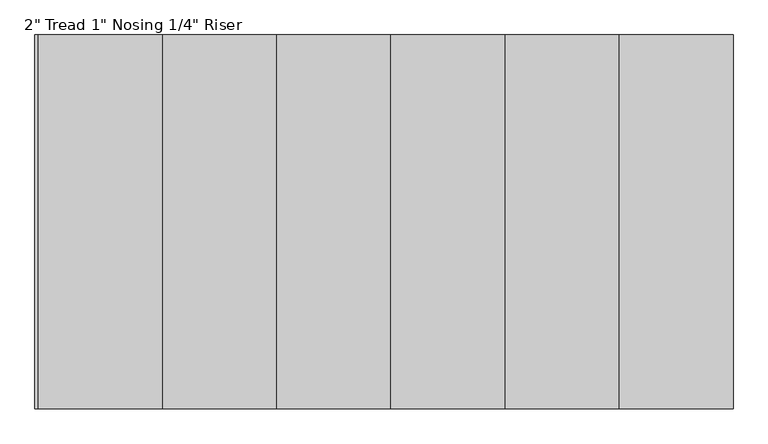
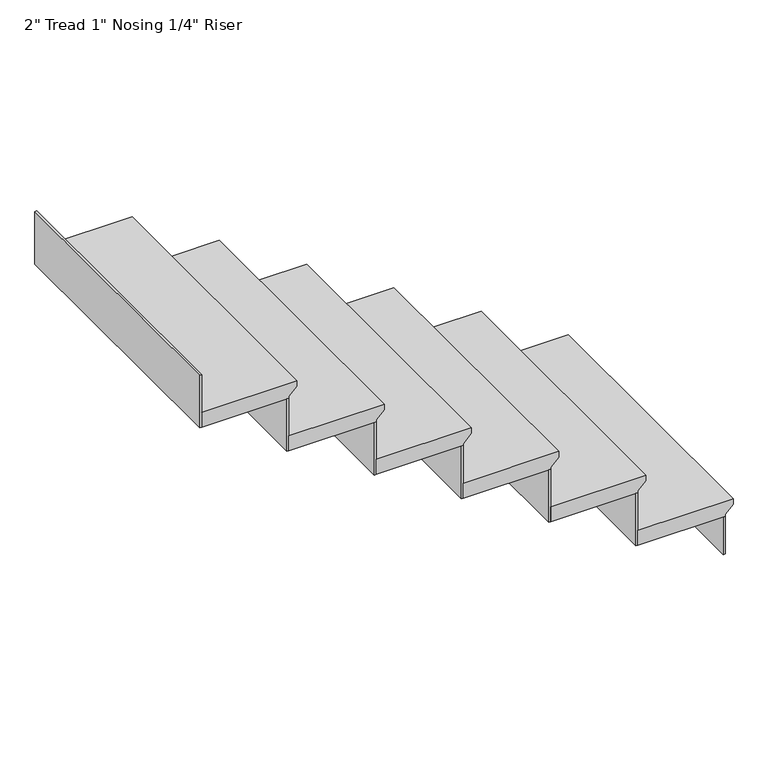
"""IFC4 building model written with IfcOpenShell, lengths in millimetres: stair flight geometry."""

from ifc_helpers import new_model, si_unit, origin, place, context, project, spatial, faceted_brep, source, transform, mapped, element, save


def stair_flight_b9929406(model_context):
    return source(origin(), model_context, "Body", "Brep", [
        faceted_brep([(-6576.0763529, -1051.6338022, 7169.15), (-6576.0763529, -1051.6338022, 7188.2), (-6576.0763529, -1966.0338022, 7188.2), (-6576.0763529, -1966.0338022, 7169.15), (-6601.4763529, -1051.6338022, 7143.75), (-6601.4763529, -1966.0338022, 7143.75), (-6880.8763529, -1051.6338022, 7188.2), (-6880.8763529, -1966.0338022, 7188.2), (-6601.4763529, -1966.0338022, 7137.4), (-6880.8763529, -1966.0338022, 7137.4), (-6880.8763529, -1051.6338022, 7137.4), (-6601.4763529, -1051.6338022, 7137.4)], [[[0, 1, 2, 3]], [[4, 0, 3, 5]], [[2, 1, 6, 7]], [[8, 9, 10, 11]], [[2, 7, 9, 8, 5, 3]], [[8, 11, 4, 5]], [[6, 1, 0, 4, 11, 10]], [[7, 6, 10, 9]]]),
        faceted_brep([(-6601.4763529, -1051.6338022, 7137.4), (-6601.4763529, -1051.6338022, 7010.4), (-6607.8263529, -1051.6338022, 7010.4), (-6607.8263529, -1051.6338022, 7137.4), (-6601.4763529, -1966.0338022, 7137.4), (-6607.8263529, -1966.0338022, 7137.4), (-6607.8263529, -1966.0338022, 7010.4), (-6601.4763529, -1966.0338022, 7010.4)], [[[0, 1, 2, 3]], [[4, 5, 6, 7]], [[1, 0, 4, 7]], [[2, 1, 7, 6]], [[3, 2, 6, 5]], [[0, 3, 5, 4]]]),
        faceted_brep([(-6880.8763529, -1051.6338022, 7315.2), (-6880.8763529, -1051.6338022, 7137.4), (-6887.2263529, -1051.6338022, 7137.4), (-6887.2263529, -1051.6338022, 7315.2), (-6880.8763529, -1966.0338022, 7315.2), (-6887.2263529, -1966.0338022, 7315.2), (-6887.2263529, -1966.0338022, 7137.4), (-6880.8763529, -1966.0338022, 7137.4)], [[[0, 1, 2, 3]], [[4, 5, 6, 7]], [[1, 0, 4, 7]], [[2, 1, 7, 6]], [[3, 2, 6, 5]], [[0, 3, 5, 4]]]),
        faceted_brep([(-6855.4763529, -1966.0338022, 7366.0), (-6855.4763529, -1051.6338022, 7366.0), (-7160.2763529, -1051.6338022, 7366.0), (-7160.2763529, -1966.0338022, 7366.0), (-6880.8763529, -1966.0338022, 7315.2), (-7160.2763529, -1966.0338022, 7315.2), (-7160.2763529, -1051.6338022, 7315.2), (-6880.8763529, -1051.6338022, 7315.2), (-6880.8763529, -1966.0338022, 7321.55), (-6855.4763529, -1966.0338022, 7346.95), (-6880.8763529, -1051.6338022, 7321.55), (-6855.4763529, -1051.6338022, 7346.95)], [[[0, 1, 2, 3]], [[4, 5, 6, 7]], [[0, 3, 5, 4, 8, 9]], [[4, 7, 10, 8]], [[2, 1, 11, 10, 7, 6]], [[3, 2, 6, 5]], [[11, 1, 0, 9]], [[10, 11, 9, 8]]]),
        faceted_brep([(-7160.2763529, -1051.6338022, 7493.0), (-7160.2763529, -1051.6338022, 7315.2), (-7166.6263529, -1051.6338022, 7315.2), (-7166.6263529, -1051.6338022, 7493.0), (-7160.2763529, -1966.0338022, 7493.0), (-7166.6263529, -1966.0338022, 7493.0), (-7166.6263529, -1966.0338022, 7315.2), (-7160.2763529, -1966.0338022, 7315.2)], [[[0, 1, 2, 3]], [[4, 5, 6, 7]], [[1, 0, 4, 7]], [[2, 1, 7, 6]], [[3, 2, 6, 5]], [[0, 3, 5, 4]]]),
        faceted_brep([(-7134.8763529, -1966.0338022, 7543.8), (-7134.8763529, -1051.6338022, 7543.8), (-7439.6763529, -1051.6338022, 7543.8), (-7439.6763529, -1966.0338022, 7543.8), (-7160.2763529, -1966.0338022, 7493.0), (-7439.6763529, -1966.0338022, 7493.0), (-7439.6763529, -1051.6338022, 7493.0), (-7160.2763529, -1051.6338022, 7493.0), (-7160.2763529, -1966.0338022, 7499.35), (-7134.8763529, -1966.0338022, 7524.75), (-7160.2763529, -1051.6338022, 7499.35), (-7134.8763529, -1051.6338022, 7524.75)], [[[0, 1, 2, 3]], [[4, 5, 6, 7]], [[0, 3, 5, 4, 8, 9]], [[4, 7, 10, 8]], [[2, 1, 11, 10, 7, 6]], [[3, 2, 6, 5]], [[11, 1, 0, 9]], [[10, 11, 9, 8]]]),
        faceted_brep([(-7439.6763529, -1051.6338022, 7670.8), (-7439.6763529, -1051.6338022, 7493.0), (-7446.0263529, -1051.6338022, 7493.0), (-7446.0263529, -1051.6338022, 7670.8), (-7439.6763529, -1966.0338022, 7670.8), (-7446.0263529, -1966.0338022, 7670.8), (-7446.0263529, -1966.0338022, 7493.0), (-7439.6763529, -1966.0338022, 7493.0)], [[[0, 1, 2, 3]], [[4, 5, 6, 7]], [[1, 0, 4, 7]], [[2, 1, 7, 6]], [[3, 2, 6, 5]], [[0, 3, 5, 4]]]),
        faceted_brep([(-7414.2763529, -1966.0338022, 7721.6), (-7414.2763529, -1051.6338022, 7721.6), (-7719.0763529, -1051.6338022, 7721.6), (-7719.0763529, -1966.0338022, 7721.6), (-7439.6763529, -1966.0338022, 7670.8), (-7719.0763529, -1966.0338022, 7670.8), (-7719.0763529, -1051.6338022, 7670.8), (-7439.6763529, -1051.6338022, 7670.8), (-7439.6763529, -1966.0338022, 7677.15), (-7414.2763529, -1966.0338022, 7702.55), (-7439.6763529, -1051.6338022, 7677.15), (-7414.2763529, -1051.6338022, 7702.55)], [[[0, 1, 2, 3]], [[4, 5, 6, 7]], [[0, 3, 5, 4, 8, 9]], [[4, 7, 10, 8]], [[2, 1, 11, 10, 7, 6]], [[3, 2, 6, 5]], [[11, 1, 0, 9]], [[10, 11, 9, 8]]]),
        faceted_brep([(-7719.0763529, -1051.6338022, 7848.6), (-7719.0763529, -1051.6338022, 7670.8), (-7725.4263529, -1051.6338022, 7670.8), (-7725.4263529, -1051.6338022, 7848.6), (-7719.0763529, -1966.0338022, 7848.6), (-7725.4263529, -1966.0338022, 7848.6), (-7725.4263529, -1966.0338022, 7670.8), (-7719.0763529, -1966.0338022, 7670.8)], [[[0, 1, 2, 3]], [[4, 5, 6, 7]], [[1, 0, 4, 7]], [[2, 1, 7, 6]], [[3, 2, 6, 5]], [[0, 3, 5, 4]]]),
        faceted_brep([(-7693.6763529, -1966.0338022, 7899.4), (-7693.6763529, -1051.6338022, 7899.4), (-7998.4763529, -1051.6338022, 7899.4), (-7998.4763529, -1966.0338022, 7899.4), (-7719.0763529, -1966.0338022, 7848.6), (-7998.4763529, -1966.0338022, 7848.6), (-7998.4763529, -1051.6338022, 7848.6), (-7719.0763529, -1051.6338022, 7848.6), (-7719.0763529, -1966.0338022, 7854.95), (-7693.6763529, -1966.0338022, 7880.35), (-7719.0763529, -1051.6338022, 7854.95), (-7693.6763529, -1051.6338022, 7880.35)], [[[0, 1, 2, 3]], [[4, 5, 6, 7]], [[0, 3, 5, 4, 8, 9]], [[4, 7, 10, 8]], [[2, 1, 11, 10, 7, 6]], [[3, 2, 6, 5]], [[11, 1, 0, 9]], [[10, 11, 9, 8]]]),
        faceted_brep([(-8277.8763529, -1051.6338022, 8204.2), (-8277.8763529, -1051.6338022, 8026.4), (-8284.2263529, -1051.6338022, 8026.4), (-8284.2263529, -1051.6338022, 8204.2), (-8277.8763529, -1966.0338022, 8204.2), (-8284.2263529, -1966.0338022, 8204.2), (-8284.2263529, -1966.0338022, 8026.4), (-8277.8763529, -1966.0338022, 8026.4)], [[[0, 1, 2, 3]], [[4, 5, 6, 7]], [[1, 0, 4, 7]], [[2, 1, 7, 6]], [[3, 2, 6, 5]], [[0, 3, 5, 4]]]),
        faceted_brep([(-7998.4763529, -1051.6338022, 8026.4), (-7998.4763529, -1051.6338022, 7848.6), (-8004.8263529, -1051.6338022, 7848.6), (-8004.8263529, -1051.6338022, 8026.4), (-7998.4763529, -1966.0338022, 8026.4), (-8004.8263529, -1966.0338022, 8026.4), (-8004.8263529, -1966.0338022, 7848.6), (-7998.4763529, -1966.0338022, 7848.6)], [[[0, 1, 2, 3]], [[4, 5, 6, 7]], [[1, 0, 4, 7]], [[2, 1, 7, 6]], [[3, 2, 6, 5]], [[0, 3, 5, 4]]]),
        faceted_brep([(-7973.0763529, -1966.0338022, 8077.2), (-7973.0763529, -1051.6338022, 8077.2), (-8252.4763529, -1051.6338022, 8077.2), (-8277.8763529, -1051.6338022, 8077.2), (-8277.8763529, -1966.0338022, 8077.2), (-7998.4763529, -1966.0338022, 8026.4), (-8277.8763529, -1966.0338022, 8026.4), (-8277.8763529, -1051.6338022, 8026.4), (-8252.4763529, -1051.6338022, 8026.4), (-7998.4763529, -1051.6338022, 8026.4), (-7998.4763529, -1966.0338022, 8032.75), (-7973.0763529, -1966.0338022, 8058.15), (-7998.4763529, -1051.6338022, 8032.75), (-7973.0763529, -1051.6338022, 8058.15)], [[[0, 1, 2, 3, 4]], [[5, 6, 7, 8, 9]], [[0, 4, 6, 5, 10, 11]], [[5, 9, 12, 10]], [[2, 1, 13, 12, 9, 8]], [[3, 2, 8, 7]], [[4, 3, 7, 6]], [[13, 1, 0, 11]], [[12, 13, 11, 10]]]),
    ])


if __name__ == "__main__":
    model = new_model("IFC4")
    model_context = context("Model", 3, world=origin())
    ifc_project = project(units=[si_unit("LENGTHUNIT", "METRE", prefix="MILLI")], contexts=[model_context])
    site = spatial("IfcSite", under=ifc_project)
    building = spatial("IfcBuilding", under=site)
    placement = place(None, origin())
    stair_flight_shape = stair_flight_b9929406(model_context)
    element("IfcStairFlight", 1, ObjectType="2\" Tread 1\" Nosing 1/4\" Riser", at=placement, inside=building, context=model_context, shape_type="MappedRepresentation", body=[
        mapped(stair_flight_shape, transform((0.0, 0.0, 0.0), x_axis=(1.0, 0.0, 0.0), y_axis=(0.0, 1.0, 0.0), z_axis=(0.0, 0.0, 1.0))),
    ])
    save(model, "model.ifc")
